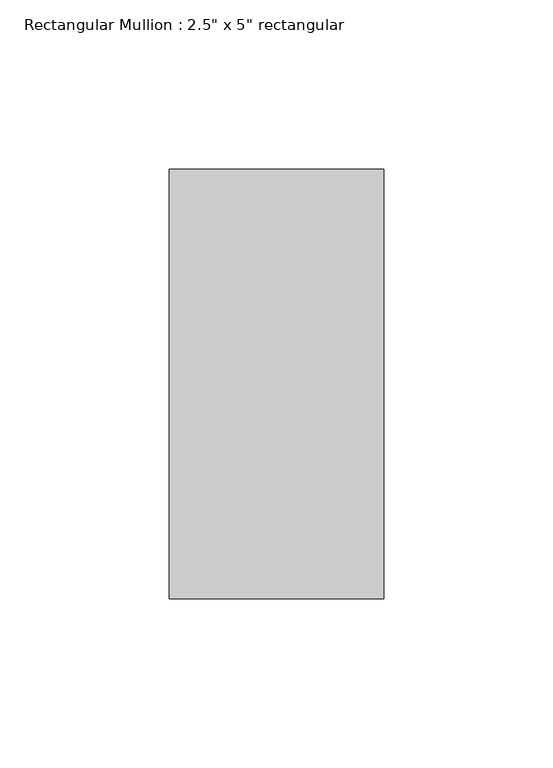
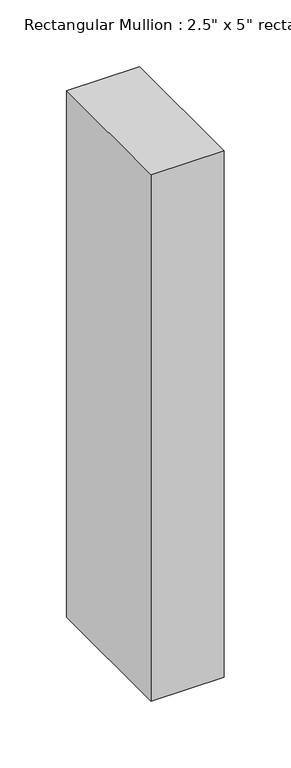
"""IFC4 building model written with IfcOpenShell, lengths in millimetres: member geometry."""

from ifc_helpers import new_model, si_unit, frame, origin, place, context, project, spatial, polyline, outline, extrude, source, transform, mapped, element, save


def member_323df77c(model_context):
    return source(origin(), model_context, "Body", "SweptSolid", [
        extrude(outline(polyline([(31.75, 63.5), (31.75, -63.5), (-31.75, -63.5), (-31.75, 63.5), (31.75, 63.5)])), frame((0.0, 0.0, -482.6), z_axis=(0.0, 0.0, 1.0), x_axis=(1.0, 0.0, 0.0)), (0.0, 0.0, 1.0), 482.6),
    ])


if __name__ == "__main__":
    model = new_model("IFC4")
    model_context = context("Model", 3, world=origin())
    ifc_project = project(units=[si_unit("LENGTHUNIT", "METRE", prefix="MILLI")], contexts=[model_context])
    site = spatial("IfcSite", under=ifc_project)
    building = spatial("IfcBuilding", under=site)
    placement = place(None, origin())
    member_shape = member_323df77c(model_context)
    element("IfcMember", 1, ObjectType="Rectangular Mullion : 2.5\" x 5\" rectangular", at=placement, inside=building, context=model_context, shape_type="MappedRepresentation", body=[
        mapped(member_shape, transform((0.0, 0.0, 0.0), x_axis=(1.0, 0.0, 0.0), y_axis=(0.0, 1.0, 0.0), z_axis=(0.0, 0.0, 1.0))),
    ])
    save(model, "model.ifc")

# Revit data of these elements
# Type "Rectangular Mullion : 2.5\" x 5\" rectangular"
#   built-in parameter 1007304 = 0.416667 (stored number, unit not read)
#   built-in parameter 1007301 = 0.104167 (stored number, unit not read)
#   built-in parameter 1007300 = 0.104167 (stored number, unit not read)
# Element 1 (IfcMember, "Rectangular Mullion : 2.5\" x 5\" rectangular")
#   Materials on its faces: "Aluminum"
# Materials
#   "Aluminum": class "Metal", colour RGB 247 247 247, transparency 0, Description = "Aluminum 6061", Cost = 0
